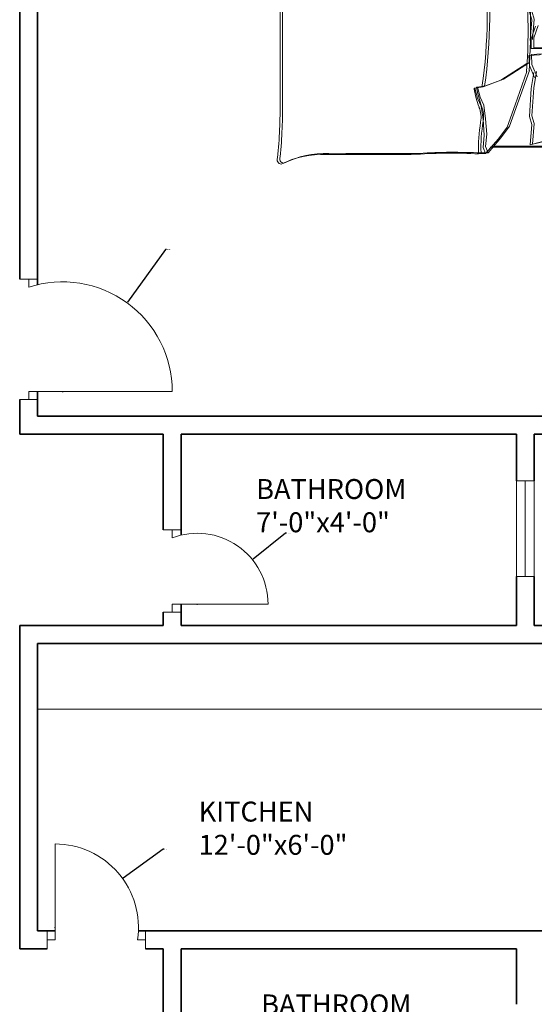
# Model space of a CAD drawing. Units: inches. Extents: x 2163 to 2982, y 1024 to 2288.
# Tile 7 of 22: x 2714 to 2843, y 1390 to 1637. Entities that reach past the tile are written whole.
import ezdxf

# ---------------------------------------------------------------- set-up
doc = ezdxf.new("R2010")
doc.units = ezdxf.units.IN
for name, color, linetype, lineweight in [('A-ANNO-DIMS', 2, 'Continuous', 18), ('A-AREA-IDEN', 7, 'Continuous', 18), ('A-DOOR', 11, 'Continuous', 18), ('A-FLOR-FIXT', 9, 'Continuous', 18), ('A-FURN', 8, 'Continuous', 13), ('A-GLAZ', 161, 'Continuous', 18), ('A-WALL', 7, 'Continuous', 35)]:
    doc.layers.add(name, color=color, linetype=linetype, lineweight=lineweight)
doc.styles.get("Standard").update_dxf_attribs({"font": 'arial.ttf'})
doc.dimstyles.get("Standard").update_dxf_attribs({"dimtxt": 0.18, "dimasz": 0.18, "dimexe": 0.18, "dimexo": 0.0625, "dimgap": 0.09, "dimtad": 0, "dimtih": 1, "dimtoh": 1, "dimdec": 4, "dimzin": 0, "dimdsep": 46, "dimtxsty": 'Standard', "dimcen": 0.09, "dimadec": 0, "dimazin": 0, "dimtfac": 1, "dimtdec": 4, "dimtofl": 0, "dimtmove": 0, "dimatfit": 3, "dimfxl": 1, "dimtolj": 1, "dimtzin": 0, "dimarcsym": 0})

# ---------------------------------------------------------------- blocks, each defined once
blk = doc.blocks.new('BED-DOUBLE')
for p, q in [((27.75, 52.87), (24.5, 49.16)), ((27.75, 52.87), (24.5, 49.16)), ((28.38, 53.1), (25.13, 49.39)), ((28.38, 53.1), (25.13, 49.39)), ((29.49, 52.95), (27.75, 52.87, 3.87)), ((29.49, 52.95), (27.75, 52.87, 3.87)), ((28.36, 51.33), (27.75, 52.87)), ((28.36, 51.33), (27.75, 52.87)), ((30.13, 53.18), (28.38, 53.1, 3.87)), ((29, 51.56), (28.38, 53.1)), ((30.13, 53.18), (28.38, 53.1, 3.87)), ((29, 51.56), (28.38, 53.1)), ((0, 51.49), (0.64, 51.49)), ((0, 3.47), (0, 51.49)), ((0, 51.27), (26.61, 51.27)), ((0, 51.27), (26.61, 51.27)), ((0.64, 51.49), (27.25, 51.49)), ((0.64, 51.49), (27.25, 51.49)), ((1.53, 3.48), (1.53, 51.27)), ((1.53, 3.47), (1.53, 51.27)), ((2.17, 3.7), (2.17, 51.49)), ((2.17, 3.7), (2.17, 51.49)), ((2.56, 50.11), (2.46, 44.71)), ((2.56, 50.11), (2.46, 44.71)), ((2.56, 50.11), (5.77, 49.73)), ((2.56, 50.11), (5.77, 49.73)), ((3.2, 50.34), (3.1, 44.94)), ((3.2, 50.34), (3.1, 44.94)), ((3.2, 50.34), (6.41, 49.96)), ((3.2, 50.34), (6.41, 49.96)), ((5.77, 49.73), (8.34, 50.33)), ((5.77, 49.73), (8.34, 50.33)), ((8.9, 49.54), (6.22, 48.36)), ((8.9, 49.54), (6.22, 48.36)), ((6.41, 49.96), (8.98, 50.56)), ((6.41, 49.96), (8.98, 50.56)), ((11.83, 50.11), (8.26, 49.31)), ((11.83, 50.11), (8.26, 49.31)), ((8.34, 50.33), (9.38, 49.81)), ((8.34, 50.33), (9.38, 49.81)), ((12.47, 50.34), (8.9, 49.54)), ((12.47, 50.34), (8.9, 49.54)), ((8.98, 50.56), (10.02, 50.04)), ((8.98, 50.56), (10.02, 50.04)), ((13.43, 49.92), (11.83, 50.11)), ((13.43, 49.92), (11.83, 50.11)), ((14.07, 50.15), (12.47, 50.34)), ((14.07, 50.15), (12.47, 50.34)), ((16.57, 50.7), (13.43, 49.92)), ((16.57, 50.7), (13.43, 49.92)), ((17.21, 50.93), (14.07, 50.15)), ((17.21, 50.93), (14.07, 50.15)), ((16.17, 45.57), (16.57, 50.7)), ((16.17, 45.57), (16.57, 50.7)), ((16.81, 45.79), (17.21, 50.93)), ((16.81, 45.79), (17.21, 50.93)), ((25.13, 49.39), (22.97, 46.45)), ((25.13, 49.39), (22.97, 46.45)), ((28.06, 48.23), (28.36, 51.33)), ((28.06, 48.23), (28.36, 51.33)), ((28.69, 48.46), (29, 51.56)), ((28.69, 48.46), (29, 51.56)), ((8.26, 49.31), (5.58, 48.13)), ((8.26, 49.31), (5.58, 48.13)), ((24.5, 49.16), (22.33, 46.22)), ((24.5, 49.16), (22.33, 46.22)), ((28.36, 44.36), (28.06, 48.23)), ((28.36, 44.36), (28.06, 48.23)), ((29, 44.59), (28.69, 48.46)), ((29, 44.59), (28.69, 48.46)), ((2.46, 44.71), (2.54, 45.71)), ((2.46, 44.71), (2.54, 45.71)), ((2.54, 45.71), (3.07, 41.91)), ((2.54, 45.71), (3.07, 41.91)), ((3.1, 44.94), (3.18, 45.94)), ((3.1, 44.94), (3.18, 45.94)), ((3.18, 45.94), (3.71, 42.14)), ((3.18, 45.94), (3.71, 42.14)), ((16.73, 43.61), (16.17, 45.57)), ((16.73, 43.61), (16.17, 45.57)), ((17.37, 43.83), (16.81, 45.79)), ((17.37, 43.83), (16.81, 45.79)), ((22.33, 46.22), (20.32, 40.64)), ((22.33, 46.22), (20.32, 40.64)), ((22.97, 46.45), (20.96, 40.87)), ((22.97, 46.45), (20.96, 40.87)), ((29.47, 41.18), (29, 44.59)), ((29.47, 41.18), (29, 44.59)), ((3.71, 42.14), (5.06, 36.72)), ((3.71, 42.14), (5.06, 36.72)), ((16.29, 36.6), (16.73, 43.61)), ((16.29, 36.6), (16.73, 43.61)), ((16.93, 36.82), (17.37, 43.83)), ((16.93, 36.82), (17.37, 43.83)), ((28.83, 40.95), (28.36, 44.36)), ((28.83, 40.95), (28.36, 44.36)), ((3.07, 41.91), (4.42, 36.49)), ((3.07, 41.91), (4.42, 36.49)), ((20.32, 40.64), (17.38, 32.31)), ((20.32, 40.64), (17.38, 32.31)), ((20.96, 40.87), (18.02, 32.53)), ((20.96, 40.87), (18.02, 32.53)), ((29.76, 38.94), (28.83, 40.95)), ((29.76, 38.94), (28.83, 40.95)), ((30.4, 39.17), (29.47, 41.18)), ((30.4, 39.17), (29.47, 41.18)), ((79.24, 15.06), (79.24, 39.68)), ((79.24, 15.06), (79.24, 39.68)), ((79.88, 15.29), (79.88, 39.91)), ((79.88, 15.29), (79.88, 39.91)), ((3.08, 37.14), (2.54, 34.2)), ((3.08, 37.13), (2.54, 34.2)), ((3.67, 39.2), (3.08, 37.14)), ((3.67, 39.2), (3.08, 37.13)), ((3.72, 37.36), (3.18, 34.43)), ((3.72, 37.36), (3.18, 34.43)), ((4.31, 39.43), (3.72, 37.36)), ((4.31, 39.43), (3.72, 37.36)), ((30.38, 36.46), (29.76, 38.94)), ((30.38, 36.46), (29.76, 38.94)), ((31.02, 36.69), (30.4, 39.17)), ((31.02, 36.69), (30.4, 39.17)), ((15.63, 32.56), (16.29, 36.6)), ((15.63, 32.56), (16.29, 36.6)), ((16.27, 32.79), (16.93, 36.82)), ((16.27, 32.79), (16.93, 36.82)), ((18.02, 30.49), (24.52, 34.68)), ((18.02, 30.49), (24.52, 34.68)), ((23.88, 34.45), (28.36, 36.15)), ((23.88, 34.45), (28.36, 36.15)), ((24.52, 34.68), (29, 36.38)), ((24.52, 34.68), (29, 36.38)), ((28.36, 36.15), (30.38, 36.46)), ((28.36, 36.15), (30.38, 36.46)), ((29, 36.38), (31.02, 36.69)), ((29, 36.38), (31.02, 36.69)), ((2.54, 34.2), (2.56, 33.88)), ((2.54, 34.2), (2.56, 33.88)), ((2.56, 33.88), (2.98, 29.46)), ((2.56, 33.88), (2.98, 29.46)), ((3.18, 34.43), (3.2, 34.11)), ((3.18, 34.43), (3.2, 34.11)), ((3.2, 34.11), (3.62, 29.68)), ((3.2, 34.11), (3.62, 29.68)), ((16.74, 30.75), (15.45, 33.82)), ((16.74, 30.75), (15.45, 33.82)), ((17.38, 30.98), (16.09, 34.05)), ((17.38, 30.98), (16.09, 34.05)), ((17.38, 30.26), (23.88, 34.45)), ((17.38, 30.26), (23.88, 34.45)), ((3.62, 29.68), (3.13, 28.21)), ((3.62, 29.68), (3.13, 28.2)), ((16.89, 28.3), (16.74, 30.75)), ((16.89, 28.3), (16.74, 30.75)), ((17.53, 28.53), (17.38, 30.98)), ((17.53, 28.53), (17.38, 30.98)), ((2.98, 29.46), (2.49, 27.98)), ((2.98, 29.46), (2.49, 27.98)), ((2.49, 27.98), (7.87, 27.73)), ((2.49, 27.98), (7.87, 27.73)), ((3.13, 28.21), (8.51, 27.96)), ((3.13, 28.2), (8.51, 27.96)), ((7.86, 26.79), (11.04, 27.37)), ((7.86, 26.79), (11.04, 27.37)), ((7.87, 27.73), (11.08, 27.35)), ((7.87, 27.73), (11.08, 27.35)), ((8.51, 27.96), (11.72, 27.58)), ((8.51, 27.96), (11.72, 27.58)), ((11.04, 27.37), (12.34, 27.37)), ((11.04, 27.37), (12.34, 27.37)), ((11.08, 27.35), (12.38, 27.44)), ((11.08, 27.35), (12.38, 27.44)), ((11.72, 27.58), (13.02, 27.66)), ((11.72, 27.58), (13.02, 27.66)), ((12.34, 27.37), (14.22, 26.79)), ((12.34, 27.37), (14.22, 26.79)), ((12.38, 27.44), (14.22, 28.13)), ((12.38, 27.44), (14.22, 28.13)), ((13.02, 27.66), (14.86, 28.36)), ((13.02, 27.66), (14.86, 28.36)), ((14.22, 28.13), (16.89, 28.3)), ((14.22, 28.13), (16.89, 28.3)), ((14.86, 28.36), (17.53, 28.53)), ((14.86, 28.36), (17.53, 28.53)), ((1.87, 25.98), (7.22, 26.56)), ((1.87, 25.98), (7.22, 26.56)), ((2.45, 24.54), (1.87, 25.98)), ((2.45, 24.54), (1.87, 25.98)), ((2.51, 26.21), (7.86, 26.79)), ((2.51, 26.21), (7.86, 26.79)), ((3.09, 24.77), (2.51, 26.21)), ((3.09, 24.77), (2.51, 26.21)), ((2.94, 20.32), (3.09, 24.77)), ((2.94, 20.32), (3.09, 24.77)), ((7.22, 26.56), (10.4, 27.14)), ((7.22, 26.56), (10.4, 27.14)), ((10.4, 27.14), (11.7, 27.14)), ((10.4, 27.14), (11.7, 27.14)), ((11.7, 27.14), (13.58, 26.56)), ((11.7, 27.14), (13.58, 26.56)), ((13.58, 26.56), (16.26, 26.56)), ((13.58, 26.56), (16.26, 26.56)), ((14.22, 26.79), (16.9, 26.79)), ((14.22, 26.79), (16.9, 26.79)), ((16.26, 26.56), (16.26, 24.1)), ((16.26, 26.56), (16.26, 24.1)), ((16.81, 19.61), (17.21, 24.74)), ((16.81, 19.61), (17.21, 24.74)), ((16.9, 26.79), (16.9, 24.33)), ((16.9, 26.79), (16.9, 24.33)), ((2.3, 20.09), (2.45, 24.54)), ((2.3, 20.09), (2.45, 24.54)), ((16.26, 24.1), (15.17, 20.96)), ((16.26, 24.1), (15.17, 20.96)), ((16.9, 24.33), (15.81, 21.19)), ((16.9, 24.33), (15.81, 21.19)), ((16.17, 19.38), (16.57, 24.52)), ((16.17, 19.38), (16.57, 24.52)), ((2.3, 19.77), (2.3, 20.09)), ((2.3, 19.77), (2.3, 20.09)), ((3.03, 16.88), (2.3, 19.77)), ((3.03, 16.88), (2.3, 19.77)), ((2.94, 20), (2.94, 20.32)), ((2.94, 20), (2.94, 20.32)), ((3.67, 17.11), (2.94, 20)), ((3.67, 17.11), (2.94, 20)), ((3.32, 12.11), (4.33, 17.6)), ((3.32, 12.11), (4.33, 17.6)), ((3.96, 12.34), (4.97, 17.83)), ((3.96, 12.34), (4.97, 17.83)), ((16.73, 17.42), (16.17, 19.38)), ((16.73, 17.42), (16.17, 19.38)), ((16.29, 10.41), (16.73, 17.42)), ((16.29, 10.41), (16.73, 17.42)), ((17.37, 17.65), (16.81, 19.61)), ((17.37, 17.65), (16.81, 19.61)), ((16.93, 10.64), (17.37, 17.65)), ((16.93, 10.64), (17.37, 17.65)), ((3.75, 14.85), (3.03, 16.88)), ((3.75, 14.85), (3.03, 16.88)), ((4.39, 15.08), (3.67, 17.11)), ((4.39, 15.08), (3.67, 17.11)), ((3.03, 8.28), (3.32, 12.11)), ((3.03, 8.28), (3.32, 12.11)), ((3.67, 8.51), (3.96, 12.34)), ((3.67, 8.51), (3.96, 12.34)), ((15.63, 6.38), (16.29, 10.41)), ((15.63, 6.38), (16.29, 10.41)), ((16.27, 6.61), (16.93, 10.64)), ((16.27, 6.61), (16.93, 10.64)), ((16.29, 10.41), (16.62, 9.28)), ((16.29, 10.41), (16.62, 9.28)), ((16.93, 10.64), (17.26, 9.51)), ((16.93, 10.64), (17.26, 9.51)), ((3.01, 8.18), (3.03, 8.28)), ((3.01, 8.18), (3.03, 8.28)), ((3.34, 3.9), (3.01, 8.18)), ((3.34, 3.9), (3.01, 8.18)), ((3.65, 8.41), (3.67, 8.51)), ((3.65, 8.41), (3.67, 8.51)), ((3.98, 4.13), (3.65, 8.41)), ((3.98, 4.13), (3.65, 8.41)), ((16.62, 9.28), (17.34, 4.18)), ((16.62, 9.28), (17.34, 4.18)), ((17.26, 9.51), (17.98, 4.41)), ((17.26, 9.51), (17.98, 4.41)), ((8.95, 5.05), (6.21, 6.06)), ((8.95, 5.05), (6.21, 6.06)), ((9.59, 5.28), (6.85, 6.29)), ((9.59, 5.28), (6.85, 6.29)), ((12.57, 4.47), (8.95, 5.05)), ((12.57, 4.47), (8.95, 5.05)), ((13.21, 4.7), (9.59, 5.28)), ((13.21, 4.7), (9.59, 5.28)), ((14.8, 4.99), (13.21, 4.7)), ((14.8, 4.99), (13.21, 4.7)), ((17.98, 4.41), (14.8, 4.99)), ((17.98, 4.41), (14.8, 4.99)), ((18.11, 3.48), (0, 3.48)), ((18.11, 3.47), (0, 3.47)), ((18.75, 3.7), (0.64, 3.7)), ((18.75, 3.7), (0.64, 3.7)), ((3.32, 3.89), (6.5, 4.47)), ((3.32, 3.89), (6.5, 4.47)), ((3.96, 4.12), (7.14, 4.7)), ((3.96, 4.12), (7.14, 4.7)), ((6.5, 4.47), (9.1, 4.04)), ((6.5, 4.47), (9.1, 4.04)), ((7.14, 4.7), (9.74, 4.27)), ((7.14, 4.7), (9.74, 4.27)), ((9.1, 4.04), (10.11, 4.62)), ((9.1, 4.04), (10.11, 4.62)), ((9.74, 4.27), (10.75, 4.85)), ((9.74, 4.27), (10.75, 4.85)), ((14.16, 4.76), (12.57, 4.47)), ((14.16, 4.76), (12.57, 4.47)), ((17.34, 4.18), (14.16, 4.76)), ((17.34, 4.18), (14.16, 4.76))]:
    blk.add_line(p, q)
for centre, radius, start, end in [((68.67, 76.16), 23.07, 267.4714, 296.4681), ((68.67, 76.16), 23.07, 267.4714, 296.4681), ((69.31, 76.39), 23.07, 267.4714, 296.4681), ((69.31, 76.39), 23.07, 267.4714, 296.4681), ((78.87, 54.41), 1.1, 332.6588, 86.02), ((78.87, 54.41), 1.1, 332.6588, 86.02), ((79.51, 54.64), 1.1, 332.6588, 86.02), ((79.51, 54.64), 1.1, 332.6588, 86.02), ((-6.66, 51.33), 36.18, 349.8763, 2.5657), ((-6.66, 51.33), 36.18, 349.8763, 2.5657), ((36.31, 182.27), 129.5, 266.9791, 273.8365), ((36.31, 182.27), 129.5, 266.9791, 273.8365), ((-6.02, 51.56), 36.18, 349.8763, 2.5657), ((-6.02, 51.56), 36.18, 349.8763, 2.5657), ((36.95, 182.49), 129.5, 266.9791, 273.8365), ((36.95, 182.49), 129.5, 266.9791, 273.8365), ((67.82, -4508.74), 4561.86, 90.00217, 90.28689), ((67.82, -4508.74), 4561.86, 90.00217, 90.28689), ((68.46, -4508.52), 4561.86, 90.00217, 90.28689), ((68.46, -4508.52), 4561.86, 90.00217, 90.28689), ((212.28, 41.15), 133.04, 174.4998, 180.6351), ((212.28, 41.15), 133.04, 174.4998, 180.6351), ((212.92, 41.38), 133.04, 174.4998, 180.6351), ((212.92, 41.38), 133.04, 174.4998, 180.6351), ((35.07, 43.74), 6.22, 168.6608, 203.7384), ((35.07, 43.74), 6.22, 168.6608, 203.7384), ((35.71, 43.97), 6.22, 168.6608, 203.7384), ((35.71, 43.97), 6.22, 168.6608, 203.7384), ((1.48, 31.15), 29.65, 10.6617, 19.8806), ((1.48, 31.15), 29.65, 10.6617, 19.8806), ((2.12, 31.38), 29.65, 10.6617, 19.8806), ((2.12, 31.38), 29.65, 10.6617, 19.8806), ((156.32, 17.76), 129.02, 171.7845, 186.9006), ((156.32, 17.76), 129.02, 171.7845, 186.9006), ((156.96, 17.98), 129.02, 171.7845, 186.9006), ((156.96, 17.98), 129.02, 171.7845, 186.9006), ((30.44, 36.64), 0.185, 250.2464, 1.1377), ((30.44, 36.64), 0.185, 250.2464, 1.1377), ((31.08, 36.86), 0.185, 250.2464, 1.1377), ((31.08, 36.86), 0.185, 250.2464, 1.1377), ((182.05, 21.36), 164.97, 176.0865, 186.7821), ((182.05, 21.36), 164.97, 176.0865, 186.7821), ((182.69, 21.59), 164.97, 176.0865, 186.7821), ((182.69, 21.59), 164.97, 176.0865, 186.7821), ((-23.71, -17.22), 106.46, 13.3832, 17.7053), ((-23.71, -17.22), 106.46, 13.3832, 17.7053), ((-23.07, -16.99), 106.46, 13.3832, 17.7053), ((-23.07, -16.99), 106.46, 13.3832, 17.7053), ((200.84, 21.43), 121.76, 182.9958, 189.4091), ((200.84, 21.43), 121.76, 182.9958, 189.4091), ((201.48, 21.66), 121.76, 182.9958, 189.4091), ((201.48, 21.65), 121.76, 182.9958, 189.4091), ((20.74, 85.39), 83.31, 268.7218, 275.604), ((20.74, 85.39), 83.31, 268.7218, 275.604), ((31.17, -167.31), 170.11, 88.4762, 91.0082), ((31.17, -167.31), 170.11, 88.4762, 91.0082), ((31.81, -167.08), 170.11, 88.4762, 91.0082), ((31.81, -167.08), 170.11, 88.4762, 91.0082), ((50.61, 484.82), 482.31, 268.2277, 271.7185), ((50.61, 484.82), 482.31, 268.2277, 271.7185), ((51.25, 485.05), 482.31, 268.2277, 271.7185), ((51.25, 485.05), 482.31, 268.2277, 271.7185), ((64.51, -26.9), 29.63, 76.0648, 88.9113), ((64.51, -26.9), 29.63, 76.0648, 88.9113), ((65.15, -26.67), 29.63, 76.0648, 88.9113), ((65.15, -26.67), 29.63, 76.0648, 88.9113), ((20.1, 85.16), 83.31, 268.7218, 275.604), ((20.1, 85.16), 83.31, 268.7218, 275.604), ((70.28, -21.66), 23.56, 67.9751, 86.652), ((70.28, -21.66), 23.56, 67.9751, 86.652), ((70.91, -21.43), 23.56, 67.9751, 86.652), ((70.91, -21.43), 23.56, 67.9751, 86.652), ((79.72, 1.09), 1.09, 236.1736, 23.4781), ((79.72, 1.09), 1.09, 236.1736, 23.4781), ((80.36, 1.32), 1.09, 236.1736, 23.4781), ((80.36, 1.32), 1.09, 236.1736, 23.4781)]:
    blk.add_arc(centre, radius, start, end)
blk = doc.blocks.new('WIN-24')
for p, q in [((0, 24), (4.5, 24)), ((0, 24), (0, 0)), ((4.5, 24), (2.25, 24)), ((2.25, 24), (2.25, 0)), ((4.5, 24), (4.5, 0)), ((2.25, 0), (0, 0)), ((0, 0), (4.5, 0))]:
    blk.add_line(p, q)
blk = doc.blocks.new('*D46')
at = {"layer": 'A-ANNO-DIMS', "color": 0, "lineweight": -2, "transparency": 16777216}
for p, q in [((2750.93, 1579.54), (2741.35, 1566.34)), ((2751.11, 1579.54), (2750.93, 1579.54)), ((2725.02, 1543.96), (2725.2, 1543.96)), ((2725.11, 1543.87), (2725.11, 1544.05))]:
    blk.add_line(p, q, dxfattribs=at)
at = {"layer": 'A-ANNO-DIMS', "color": 0, "transparency": 16777216}
blk.add_solid([(2741.33, 1566.36), (2741.38, 1566.32), (2741.25, 1566.19)], dxfattribs=at)
at = {"layer": 'Defpoints', "color": 0, "transparency": 16777216}
for p in [(2741.25, 1566.19), (2725.11, 1543.96)]:
    blk.add_point(p, dxfattribs=at)
at = {"layer": 'A-ANNO-DIMS', "color": 0, "transparency": 16777216, "insert": (2751.66, 1579.54), "char_height": 0.18, "attachment_point": 5}
blk.add_mtext('\\A1;R27.475', dxfattribs=at)
blk = doc.blocks.new('*D76')
at = {"layer": 'A-ANNO-DIMS', "color": 0, "lineweight": -2, "transparency": 16777216}
for p, q in [((2750.34, 1429.18), (2740.31, 1421.95)), ((2750.52, 1429.18), (2750.34, 1429.18)), ((2723.12, 1409.6), (2723.3, 1409.6)), ((2723.21, 1409.51), (2723.21, 1409.69))]:
    blk.add_line(p, q, dxfattribs=at)
at = {"layer": 'A-ANNO-DIMS', "color": 0, "transparency": 16777216}
blk.add_solid([(2740.29, 1421.97), (2740.33, 1421.92), (2740.17, 1421.84)], dxfattribs=at)
at = {"layer": 'Defpoints', "color": 0, "transparency": 16777216}
for p in [(2740.17, 1421.84), (2723.21, 1409.6)]:
    blk.add_point(p, dxfattribs=at)
at = {"layer": 'A-ANNO-DIMS', "color": 0, "transparency": 16777216, "insert": (2751.07, 1429.18), "char_height": 0.18, "attachment_point": 5}
blk.add_mtext('\\A1;R20.915', dxfattribs=at)
blk = doc.blocks.new('*D78')
at = {"layer": 'A-ANNO-DIMS', "color": 0, "lineweight": -2, "transparency": 16777216}
for p, q in [((2781, 1508.41), (2772.83, 1501.87)), ((2781.18, 1508.41), (2781, 1508.41)), ((2758.75, 1490.66), (2758.93, 1490.66)), ((2758.84, 1490.57), (2758.84, 1490.75))]:
    blk.add_line(p, q, dxfattribs=at)
at = {"layer": 'A-ANNO-DIMS', "color": 0, "transparency": 16777216}
blk.add_solid([(2772.82, 1501.89), (2772.85, 1501.84), (2772.69, 1501.76)], dxfattribs=at)
at = {"layer": 'Defpoints', "color": 0, "transparency": 16777216}
for p in [(2772.69, 1501.76), (2758.84, 1490.66)]:
    blk.add_point(p, dxfattribs=at)
at = {"layer": 'A-ANNO-DIMS', "color": 0, "transparency": 16777216, "insert": (2781.74, 1508.41), "char_height": 0.18, "attachment_point": 5}
blk.add_mtext('\\A1;R17.745', dxfattribs=at)

msp = doc.modelspace()

# ---------------------------------------------------------------- linework, layer by layer
at = {"layer": 'A-DOOR'}
for p, q in [((2718.8389, 1572.0744), (2714.3389, 1572.0744)), ((2714.3389, 1572.0744), (2716.5889, 1572.0744)), ((2716.5889, 1572.0744), (2716.5889, 1570.0744)), ((2716.5889, 1541.955), (2716.5889, 1543.955)), ((2716.5889, 1543.955), (2752.5889, 1543.955)), ((2714.3389, 1541.955), (2718.8389, 1541.955)), ((2718.8389, 1541.955), (2716.5889, 1541.955)), ((2750.3389, 1509.2688), (2754.8389, 1509.2688)), ((2754.8389, 1509.2688), (2752.5889, 1509.2688)), ((2752.5889, 1509.2688), (2752.5889, 1507.2688)), ((2750.3389, 1488.6623), (2754.8389, 1488.6623)), ((2752.5889, 1488.6623), (2752.5889, 1490.6623)), ((2752.5889, 1490.6623), (2776.5889, 1490.6623)), ((2754.8389, 1488.6623), (2752.5889, 1488.6623)), ((2723.2052, 1406.5188), (2723.2052, 1430.5188)), ((2721.2052, 1408.7688), (2721.2052, 1404.2688)), ((2745.8913, 1408.7688), (2745.8913, 1404.2688)), ((2721.2052, 1404.2688), (2721.2052, 1406.5188)), ((2721.2052, 1406.5188), (2723.2052, 1406.5188)), ((2745.8913, 1406.5188), (2743.8913, 1406.5188)), ((2745.8913, 1404.2688), (2745.8913, 1406.5188))]:
    msp.add_line(p, q, dxfattribs=at)
for centre, radius, start, end in [((2725.1136, 1543.955), 27.4753, 0, 108.075469), ((2758.8436, 1490.6623), 17.7453, 360, 110.638327), ((2723.2052, 1409.6039), 20.915, 351.517666, 90)]:
    msp.add_arc(centre, radius, start, end, dxfattribs=at)
at = {"layer": 'A-FLOR-FIXT'}
msp.add_line((2848.1781, 1464.335), (2718.8389, 1464.335), dxfattribs=at)
at = {"layer": 'A-WALL'}
for p, q in [((2714.3389, 1681.7688), (2714.3389, 1572.0744)), ((2718.8389, 1681.7688), (2718.8389, 1570.7042)), ((2718.8389, 1543.955), (2718.8389, 1537.7688)), ((2714.3389, 1541.955), (2714.3389, 1533.2688)), ((2718.8389, 1537.7688), (2862.8389, 1537.7688)), ((2714.3389, 1533.2688), (2750.3389, 1533.2688)), ((2750.3389, 1509.2688), (2750.3389, 1533.2688)), ((2838.8389, 1533.2688), (2754.8389, 1533.2688)), ((2754.8389, 1533.2688), (2754.8389, 1507.9499)), ((2754.8389, 1533.2688), (2838.8389, 1533.2688)), ((2838.8389, 1533.2688), (2838.8389, 1521.5742)), ((2867.3389, 1533.2688), (2843.3389, 1533.2688)), ((2843.3389, 1533.2688), (2862.8389, 1533.2688)), ((2843.3389, 1521.5742), (2843.3389, 1533.2688)), ((2838.8389, 1497.5742), (2838.8389, 1485.2688)), ((2843.3389, 1485.2688), (2843.3389, 1497.5742)), ((2750.3389, 1485.2688), (2750.3389, 1488.6623)), ((2754.8389, 1490.6623), (2754.8389, 1485.2688)), ((2714.3389, 1485.2688), (2750.3389, 1485.2688)), ((2714.3389, 1485.2688), (2714.3389, 1404.2688)), ((2754.8389, 1485.2688), (2838.8389, 1485.2688)), ((2843.3389, 1485.2688), (2867.3389, 1485.2688)), ((2718.8389, 1480.7688), (2862.8389, 1480.7688)), ((2718.8389, 1480.7688), (2718.8389, 1408.7688)), ((2718.8389, 1408.7688), (2723.2052, 1408.7688)), ((2744.1034, 1408.7688), (2862.8389, 1408.7688)), ((2714.3389, 1404.2688), (2721.2052, 1404.2688)), ((2745.8913, 1404.2688), (2750.3389, 1404.2688)), ((2750.3389, 1404.2688), (2750.3389, 1356.2688)), ((2754.8389, 1356.2688), (2754.8389, 1404.2688)), ((2754.8389, 1404.2688), (2838.8389, 1404.2688)), ((2838.8389, 1390.3249), (2838.8389, 1404.2688))]:
    msp.add_line(p, q, dxfattribs=at)

# ---------------------------------------------------------------- block references
at = {"layer": 'A-FURN', "rotation": 180}
msp.add_blockref('BED-DOUBLE', (2859.4875, 1656.6782), dxfattribs=at)
at = {"layer": 'A-GLAZ', "extrusion": (0, 0, -1), "zscale": -1, "rotation": 180}
msp.add_blockref('WIN-24', (-2838.839, 1521.5737), dxfattribs=at)

# ---------------------------------------------------------------- texts
at = {"layer": 'A-AREA-IDEN', "char_height": 5, "attachment_point": 1}
for s, width, insert in [('BATHROOM\\P7\'-0"x4\'-0"', 55.8462, (2773.6066, 1521.9921)), ('KITCHEN\\P12\'-0"x6\'-0"', 83.391823, (2759.1866, 1441.1347)), ('BATHROOM\\P7\'-0"x4\'-0"', 52.770015, (2774.8723, 1392.7938))]:
    msp.add_mtext_dynamic_manual_height_columns(s, width=width, gutter_width=12.5, heights=[0], dxfattribs=dict(at, insert=insert))

# ---------------------------------------------------------------- dimensions: what is measured, and where the dimension line sits
at = {"layer": 'A-ANNO-DIMS'}
for center, mpoint, picture, middle in [((2725.1136, 1543.955), (2741.2487, 1566.1936), '*D46', (2751.6601, 1579.5367)), ((2758.8436, 1490.6623), (2772.6944, 1501.7552), '*D78', (2781.7353, 1508.411)), ((2723.2052, 1409.6039), (2740.1662, 1421.8414), '*D76', (2751.0733, 1429.184))]:
    dim = msp.add_radius_dim(center=center, mpoint=mpoint, dimstyle='Standard', override={"dimdec": 3, "dimlfac": 1, "dimrnd": 0, "dimzin": 0, "dimdsep": 46, "dimlunit": 2}, dxfattribs=at)
    dim.commit()
    dim.dimension.update_dxf_attribs({"geometry": picture, "text_midpoint": middle, "dimtype": 164})

doc.saveas('drawing.dxf')
